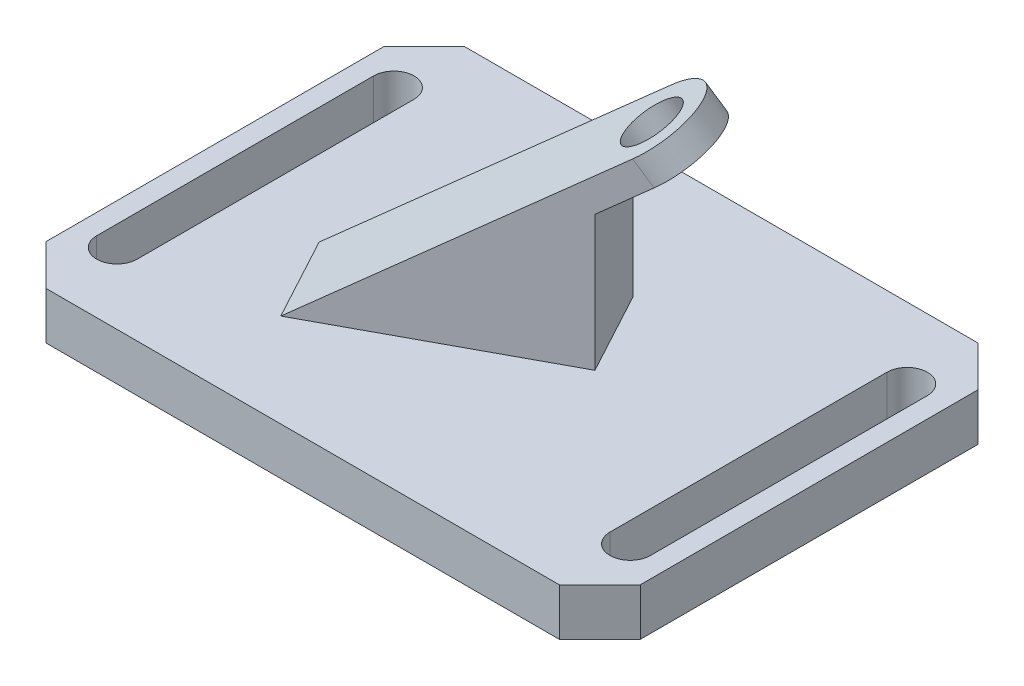
ISO-10303-21;
HEADER;
FILE_DESCRIPTION(('STEP AP214'),'2;1');
FILE_NAME('part.step','',(''),(''),'','','');
FILE_SCHEMA(('AUTOMOTIVE_DESIGN { 1 0 10303 214 1 1 1 1 }'));
ENDSEC;
DATA;
#1=APPLICATION_CONTEXT('core data for automotive mechanical design processes');
#2=APPLICATION_PROTOCOL_DEFINITION('international standard','automotive_design',2000,#1);
#3=PRODUCT_CONTEXT('',#1,'mechanical');
#4=PRODUCT('Part','Part','',(#3));
#5=PRODUCT_RELATED_PRODUCT_CATEGORY('part','',(#4));
#6=PRODUCT_DEFINITION_FORMATION('','',#4);
#7=PRODUCT_DEFINITION_CONTEXT('part definition',#1,'design');
#8=PRODUCT_DEFINITION('design','',#6,#7);
#9=PRODUCT_DEFINITION_SHAPE('','',#8);
#10=(LENGTH_UNIT() NAMED_UNIT(*) SI_UNIT(.MILLI.,.METRE.));
#11=(NAMED_UNIT(*) PLANE_ANGLE_UNIT() SI_UNIT($,.RADIAN.));
#12=(NAMED_UNIT(*) SI_UNIT($,.STERADIAN.) SOLID_ANGLE_UNIT());
#13=UNCERTAINTY_MEASURE_WITH_UNIT(LENGTH_MEASURE(1.E-05),#10,'distance_accuracy_value','');
#14=(GEOMETRIC_REPRESENTATION_CONTEXT(3) GLOBAL_UNCERTAINTY_ASSIGNED_CONTEXT((#13)) GLOBAL_UNIT_ASSIGNED_CONTEXT((#10,
#11,#12)) REPRESENTATION_CONTEXT('',''));
#15=CARTESIAN_POINT('',(0.,0.,0.));
#16=DIRECTION('',(0.,0.,1.));
#17=DIRECTION('',(1.,0.,0.));
#18=AXIS2_PLACEMENT_3D('',#15,#16,#17);
#19=CARTESIAN_POINT('',(0.,3.5,0.));
#20=DIRECTION('',(0.,-1.,0.));
#21=DIRECTION('',(0.,0.,-1.));
#22=AXIS2_PLACEMENT_3D('',#19,#20,#21);
#23=PLANE('',#22);
#24=DIRECTION('',(-0.474790242570468,0.,-0.880098986228183));
#25=VECTOR('',#24,1.);
#26=CARTESIAN_POINT('',(13.141813392465,3.5,0.863988305263869));
#27=LINE('',#26,#25);
#28=CARTESIAN_POINT('',(13.141813392465,3.5,0.863988305263869));
#29=VERTEX_POINT('',#28);
#30=CARTESIAN_POINT('',(6.49474999647841,3.5,-11.4573975019307));
#31=VERTEX_POINT('',#30);
#32=EDGE_CURVE('E59',#29,#31,#27,.T.);
#33=ORIENTED_EDGE('',*,*,#32,.F.);
#34=DIRECTION('',(0.880098986228183,0.,-0.474790242570468));
#35=VECTOR('',#34,1.);
#36=CARTESIAN_POINT('',(-17.074488577443,3.5,17.1648880521879));
#37=LINE('',#36,#35);
#38=CARTESIAN_POINT('',(-17.074488577443,3.5,17.1648880521879));
#39=VERTEX_POINT('',#38);
#40=EDGE_CURVE('E61',#39,#29,#37,.T.);
#41=ORIENTED_EDGE('',*,*,#40,.F.);
#42=DIRECTION('',(-0.474790242570468,0.,-0.880098986228183));
#43=VECTOR('',#42,1.);
#44=CARTESIAN_POINT('',(-17.074488577443,3.5,17.1648880521879));
#45=LINE('',#44,#43);
#46=CARTESIAN_POINT('',(-23.7215519734296,3.5,4.84350224499337));
#47=VERTEX_POINT('',#46);
#48=EDGE_CURVE('E228',#39,#47,#45,.T.);
#49=ORIENTED_EDGE('',*,*,#48,.T.);
#50=DIRECTION('',(0.880098986228183,0.,-0.474790242570468));
#51=VECTOR('',#50,1.);
#52=CARTESIAN_POINT('',(-23.7215519734296,3.5,4.84350224499337));
#53=LINE('',#52,#51);
#54=EDGE_CURVE('E192',#47,#31,#53,.T.);
#55=ORIENTED_EDGE('',*,*,#54,.T.);
#56=EDGE_LOOP('',(#33,#41,#49,#55));
#57=FACE_BOUND('',#56,.T.);
#58=CARTESIAN_POINT('',(-38.,3.5,20.5));
#59=DIRECTION('',(0.,1.,0.));
#60=DIRECTION('',(0.,0.,1.));
#61=AXIS2_PLACEMENT_3D('',#58,#59,#60);
#62=CIRCLE('',#61,3.);
#63=CARTESIAN_POINT('',(-41.,3.5,20.5));
#64=VERTEX_POINT('',#63);
#65=CARTESIAN_POINT('',(-35.,3.5,20.5));
#66=VERTEX_POINT('',#65);
#67=EDGE_CURVE('E268',#64,#66,#62,.T.);
#68=ORIENTED_EDGE('',*,*,#67,.F.);
#69=DIRECTION('',(0.,0.,1.));
#70=VECTOR('',#69,1.);
#71=CARTESIAN_POINT('',(-41.,3.5,20.5));
#72=LINE('',#71,#70);
#73=CARTESIAN_POINT('',(-41.,3.5,-20.5));
#74=VERTEX_POINT('',#73);
#75=EDGE_CURVE('E277',#74,#64,#72,.T.);
#76=ORIENTED_EDGE('',*,*,#75,.F.);
#77=CARTESIAN_POINT('',(-38.,3.5,-20.5));
#78=DIRECTION('',(0.,1.,0.));
#79=DIRECTION('',(0.,0.,1.));
#80=AXIS2_PLACEMENT_3D('',#77,#78,#79);
#81=CIRCLE('',#80,3.);
#82=CARTESIAN_POINT('',(-35.,3.5,-20.5));
#83=VERTEX_POINT('',#82);
#84=EDGE_CURVE('E272',#83,#74,#81,.T.);
#85=ORIENTED_EDGE('',*,*,#84,.F.);
#86=DIRECTION('',(0.,0.,-1.));
#87=VECTOR('',#86,1.);
#88=CARTESIAN_POINT('',(-35.,3.5,20.5));
#89=LINE('',#88,#87);
#90=EDGE_CURVE('E269',#66,#83,#89,.T.);
#91=ORIENTED_EDGE('',*,*,#90,.F.);
#92=EDGE_LOOP('',(#68,#76,#85,#91));
#93=FACE_BOUND('',#92,.T.);
#94=DIRECTION('',(-1.,0.,0.));
#95=VECTOR('',#94,1.);
#96=CARTESIAN_POINT('',(-38.,3.5,-31.));
#97=LINE('',#96,#95);
#98=CARTESIAN_POINT('',(38.,3.5,-31.));
#99=VERTEX_POINT('',#98);
#100=CARTESIAN_POINT('',(-38.,3.5,-31.));
#101=VERTEX_POINT('',#100);
#102=EDGE_CURVE('E299',#99,#101,#97,.T.);
#103=ORIENTED_EDGE('',*,*,#102,.T.);
#104=DIRECTION('',(-0.707106781186549,0.,0.707106781186546));
#105=VECTOR('',#104,1.);
#106=CARTESIAN_POINT('',(-44.,3.5,-25.));
#107=LINE('',#106,#105);
#108=CARTESIAN_POINT('',(-44.,3.5,-25.));
#109=VERTEX_POINT('',#108);
#110=EDGE_CURVE('E305',#101,#109,#107,.T.);
#111=ORIENTED_EDGE('',*,*,#110,.T.);
#112=DIRECTION('',(0.,0.,1.));
#113=VECTOR('',#112,1.);
#114=CARTESIAN_POINT('',(-44.,3.5,-25.));
#115=LINE('',#114,#113);
#116=CARTESIAN_POINT('',(-44.,3.5,25.));
#117=VERTEX_POINT('',#116);
#118=EDGE_CURVE('E304',#109,#117,#115,.T.);
#119=ORIENTED_EDGE('',*,*,#118,.T.);
#120=DIRECTION('',(0.707106781186547,0.,0.707106781186549));
#121=VECTOR('',#120,1.);
#122=CARTESIAN_POINT('',(-44.,3.5,25.));
#123=LINE('',#122,#121);
#124=CARTESIAN_POINT('',(-38.,3.5,31.));
#125=VERTEX_POINT('',#124);
#126=EDGE_CURVE('E307',#117,#125,#123,.T.);
#127=ORIENTED_EDGE('',*,*,#126,.T.);
#128=DIRECTION('',(1.,0.,0.));
#129=VECTOR('',#128,1.);
#130=CARTESIAN_POINT('',(-38.,3.5,31.));
#131=LINE('',#130,#129);
#132=CARTESIAN_POINT('',(38.,3.5,31.));
#133=VERTEX_POINT('',#132);
#134=EDGE_CURVE('E310',#125,#133,#131,.T.);
#135=ORIENTED_EDGE('',*,*,#134,.T.);
#136=DIRECTION('',(0.707106781186549,0.,-0.707106781186546));
#137=VECTOR('',#136,1.);
#138=CARTESIAN_POINT('',(38.,3.5,31.));
#139=LINE('',#138,#137);
#140=CARTESIAN_POINT('',(44.,3.5,25.));
#141=VERTEX_POINT('',#140);
#142=EDGE_CURVE('E313',#133,#141,#139,.T.);
#143=ORIENTED_EDGE('',*,*,#142,.T.);
#144=DIRECTION('',(0.,0.,-1.));
#145=VECTOR('',#144,1.);
#146=CARTESIAN_POINT('',(44.,3.5,-25.));
#147=LINE('',#146,#145);
#148=CARTESIAN_POINT('',(44.,3.5,-25.));
#149=VERTEX_POINT('',#148);
#150=EDGE_CURVE('E311',#141,#149,#147,.T.);
#151=ORIENTED_EDGE('',*,*,#150,.T.);
#152=DIRECTION('',(-0.707106781186549,0.,-0.707106781186547));
#153=VECTOR('',#152,1.);
#154=CARTESIAN_POINT('',(38.,3.5,-31.));
#155=LINE('',#154,#153);
#156=EDGE_CURVE('E312',#149,#99,#155,.T.);
#157=ORIENTED_EDGE('',*,*,#156,.T.);
#158=EDGE_LOOP('',(#103,#111,#119,#127,#135,#143,#151,#157));
#159=FACE_BOUND('',#158,.T.);
#160=CARTESIAN_POINT('',(38.,3.5,20.5));
#161=DIRECTION('',(0.,1.,0.));
#162=DIRECTION('',(0.,0.,-1.));
#163=AXIS2_PLACEMENT_3D('',#160,#161,#162);
#164=CIRCLE('',#163,3.);
#165=CARTESIAN_POINT('',(35.,3.5,20.5));
#166=VERTEX_POINT('',#165);
#167=CARTESIAN_POINT('',(41.,3.5,20.5));
#168=VERTEX_POINT('',#167);
#169=EDGE_CURVE('E240',#166,#168,#164,.T.);
#170=ORIENTED_EDGE('',*,*,#169,.F.);
#171=DIRECTION('',(0.,0.,1.));
#172=VECTOR('',#171,1.);
#173=CARTESIAN_POINT('',(35.,3.5,20.5));
#174=LINE('',#173,#172);
#175=CARTESIAN_POINT('',(35.,3.5,-20.5));
#176=VERTEX_POINT('',#175);
#177=EDGE_CURVE('E242',#176,#166,#174,.T.);
#178=ORIENTED_EDGE('',*,*,#177,.F.);
#179=CARTESIAN_POINT('',(38.,3.5,-20.5));
#180=DIRECTION('',(0.,1.,0.));
#181=DIRECTION('',(0.,0.,-1.));
#182=AXIS2_PLACEMENT_3D('',#179,#180,#181);
#183=CIRCLE('',#182,3.);
#184=CARTESIAN_POINT('',(41.,3.5,-20.5));
#185=VERTEX_POINT('',#184);
#186=EDGE_CURVE('E245',#185,#176,#183,.T.);
#187=ORIENTED_EDGE('',*,*,#186,.F.);
#188=DIRECTION('',(0.,0.,-1.));
#189=VECTOR('',#188,1.);
#190=CARTESIAN_POINT('',(41.,3.5,20.5));
#191=LINE('',#190,#189);
#192=EDGE_CURVE('E239',#168,#185,#191,.T.);
#193=ORIENTED_EDGE('',*,*,#192,.F.);
#194=EDGE_LOOP('',(#170,#178,#187,#193));
#195=FACE_BOUND('',#194,.T.);
#196=ADVANCED_FACE('F43',(#57,#93,#159,#195),#23,.F.);
#197=CARTESIAN_POINT('',(0.,-3.5,0.));
#198=DIRECTION('',(0.,-1.,0.));
#199=DIRECTION('',(0.,0.,-1.));
#200=AXIS2_PLACEMENT_3D('',#197,#198,#199);
#201=PLANE('',#200);
#202=DIRECTION('',(-1.,0.,0.));
#203=VECTOR('',#202,1.);
#204=CARTESIAN_POINT('',(-38.,-3.5,-31.));
#205=LINE('',#204,#203);
#206=CARTESIAN_POINT('',(38.,-3.5,-31.));
#207=VERTEX_POINT('',#206);
#208=CARTESIAN_POINT('',(-38.,-3.5,-31.));
#209=VERTEX_POINT('',#208);
#210=EDGE_CURVE('E296',#207,#209,#205,.T.);
#211=ORIENTED_EDGE('',*,*,#210,.F.);
#212=DIRECTION('',(-0.707106781186549,0.,-0.707106781186547));
#213=VECTOR('',#212,1.);
#214=CARTESIAN_POINT('',(38.,-3.5,-31.));
#215=LINE('',#214,#213);
#216=CARTESIAN_POINT('',(44.,-3.5,-25.));
#217=VERTEX_POINT('',#216);
#218=EDGE_CURVE('E302',#217,#207,#215,.T.);
#219=ORIENTED_EDGE('',*,*,#218,.F.);
#220=DIRECTION('',(0.,0.,-1.));
#221=VECTOR('',#220,1.);
#222=CARTESIAN_POINT('',(44.,-3.5,-25.));
#223=LINE('',#222,#221);
#224=CARTESIAN_POINT('',(44.,-3.5,25.));
#225=VERTEX_POINT('',#224);
#226=EDGE_CURVE('E329',#225,#217,#223,.T.);
#227=ORIENTED_EDGE('',*,*,#226,.F.);
#228=DIRECTION('',(0.707106781186549,0.,-0.707106781186546));
#229=VECTOR('',#228,1.);
#230=CARTESIAN_POINT('',(38.,-3.5,31.));
#231=LINE('',#230,#229);
#232=CARTESIAN_POINT('',(38.,-3.5,31.));
#233=VERTEX_POINT('',#232);
#234=EDGE_CURVE('E327',#233,#225,#231,.T.);
#235=ORIENTED_EDGE('',*,*,#234,.F.);
#236=DIRECTION('',(1.,0.,0.));
#237=VECTOR('',#236,1.);
#238=CARTESIAN_POINT('',(-38.,-3.5,31.));
#239=LINE('',#238,#237);
#240=CARTESIAN_POINT('',(-38.,-3.5,31.));
#241=VERTEX_POINT('',#240);
#242=EDGE_CURVE('E326',#241,#233,#239,.T.);
#243=ORIENTED_EDGE('',*,*,#242,.F.);
#244=DIRECTION('',(0.707106781186547,0.,0.707106781186549));
#245=VECTOR('',#244,1.);
#246=CARTESIAN_POINT('',(-44.,-3.5,25.));
#247=LINE('',#246,#245);
#248=CARTESIAN_POINT('',(-44.,-3.5,25.));
#249=VERTEX_POINT('',#248);
#250=EDGE_CURVE('E322',#249,#241,#247,.T.);
#251=ORIENTED_EDGE('',*,*,#250,.F.);
#252=DIRECTION('',(0.,0.,1.));
#253=VECTOR('',#252,1.);
#254=CARTESIAN_POINT('',(-44.,-3.5,-25.));
#255=LINE('',#254,#253);
#256=CARTESIAN_POINT('',(-44.,-3.5,-25.));
#257=VERTEX_POINT('',#256);
#258=EDGE_CURVE('E325',#257,#249,#255,.T.);
#259=ORIENTED_EDGE('',*,*,#258,.F.);
#260=DIRECTION('',(-0.707106781186549,0.,0.707106781186546));
#261=VECTOR('',#260,1.);
#262=CARTESIAN_POINT('',(-44.,-3.5,-25.));
#263=LINE('',#262,#261);
#264=EDGE_CURVE('E319',#209,#257,#263,.T.);
#265=ORIENTED_EDGE('',*,*,#264,.F.);
#266=EDGE_LOOP('',(#211,#219,#227,#235,#243,#251,#259,#265));
#267=FACE_BOUND('',#266,.T.);
#268=DIRECTION('',(0.,0.,1.));
#269=VECTOR('',#268,1.);
#270=CARTESIAN_POINT('',(-41.,-3.5,20.5));
#271=LINE('',#270,#269);
#272=CARTESIAN_POINT('',(-41.,-3.5,-20.5));
#273=VERTEX_POINT('',#272);
#274=CARTESIAN_POINT('',(-41.,-3.5,20.5));
#275=VERTEX_POINT('',#274);
#276=EDGE_CURVE('E271',#273,#275,#271,.T.);
#277=ORIENTED_EDGE('',*,*,#276,.T.);
#278=CARTESIAN_POINT('',(-38.,-3.5,20.5));
#279=DIRECTION('',(0.,1.,0.));
#280=DIRECTION('',(0.,0.,1.));
#281=AXIS2_PLACEMENT_3D('',#278,#279,#280);
#282=CIRCLE('',#281,3.);
#283=CARTESIAN_POINT('',(-35.,-3.5,20.5));
#284=VERTEX_POINT('',#283);
#285=EDGE_CURVE('E270',#275,#284,#282,.T.);
#286=ORIENTED_EDGE('',*,*,#285,.T.);
#287=DIRECTION('',(0.,0.,-1.));
#288=VECTOR('',#287,1.);
#289=CARTESIAN_POINT('',(-35.,-3.5,20.5));
#290=LINE('',#289,#288);
#291=CARTESIAN_POINT('',(-35.,-3.5,-20.5));
#292=VERTEX_POINT('',#291);
#293=EDGE_CURVE('E283',#284,#292,#290,.T.);
#294=ORIENTED_EDGE('',*,*,#293,.T.);
#295=CARTESIAN_POINT('',(-38.,-3.5,-20.5));
#296=DIRECTION('',(0.,1.,0.));
#297=DIRECTION('',(0.,0.,1.));
#298=AXIS2_PLACEMENT_3D('',#295,#296,#297);
#299=CIRCLE('',#298,3.);
#300=EDGE_CURVE('E284',#292,#273,#299,.T.);
#301=ORIENTED_EDGE('',*,*,#300,.T.);
#302=EDGE_LOOP('',(#277,#286,#294,#301));
#303=FACE_BOUND('',#302,.T.);
#304=DIRECTION('',(0.,0.,1.));
#305=VECTOR('',#304,1.);
#306=CARTESIAN_POINT('',(35.,-3.5,20.5));
#307=LINE('',#306,#305);
#308=CARTESIAN_POINT('',(35.,-3.5,-20.5));
#309=VERTEX_POINT('',#308);
#310=CARTESIAN_POINT('',(35.,-3.5,20.5));
#311=VERTEX_POINT('',#310);
#312=EDGE_CURVE('E238',#309,#311,#307,.T.);
#313=ORIENTED_EDGE('',*,*,#312,.T.);
#314=CARTESIAN_POINT('',(38.,-3.5,20.5));
#315=DIRECTION('',(0.,1.,0.));
#316=DIRECTION('',(0.,0.,-1.));
#317=AXIS2_PLACEMENT_3D('',#314,#315,#316);
#318=CIRCLE('',#317,3.);
#319=CARTESIAN_POINT('',(41.,-3.5,20.5));
#320=VERTEX_POINT('',#319);
#321=EDGE_CURVE('E237',#311,#320,#318,.T.);
#322=ORIENTED_EDGE('',*,*,#321,.T.);
#323=DIRECTION('',(0.,0.,-1.));
#324=VECTOR('',#323,1.);
#325=CARTESIAN_POINT('',(41.,-3.5,20.5));
#326=LINE('',#325,#324);
#327=CARTESIAN_POINT('',(41.,-3.5,-20.5));
#328=VERTEX_POINT('',#327);
#329=EDGE_CURVE('E249',#320,#328,#326,.T.);
#330=ORIENTED_EDGE('',*,*,#329,.T.);
#331=CARTESIAN_POINT('',(38.,-3.5,-20.5));
#332=DIRECTION('',(0.,1.,0.));
#333=DIRECTION('',(0.,0.,-1.));
#334=AXIS2_PLACEMENT_3D('',#331,#332,#333);
#335=CIRCLE('',#334,3.);
#336=EDGE_CURVE('E251',#328,#309,#335,.T.);
#337=ORIENTED_EDGE('',*,*,#336,.T.);
#338=EDGE_LOOP('',(#313,#322,#330,#337));
#339=FACE_BOUND('',#338,.T.);
#340=ADVANCED_FACE('F359',(#267,#303,#339),#201,.T.);
#341=CARTESIAN_POINT('',(-38.,3.5,-31.));
#342=DIRECTION('',(0.,0.,1.));
#343=DIRECTION('',(1.,0.,0.));
#344=AXIS2_PLACEMENT_3D('',#341,#342,#343);
#345=PLANE('',#344);
#346=ORIENTED_EDGE('',*,*,#210,.T.);
#347=DIRECTION('',(0.,-1.,0.));
#348=VECTOR('',#347,1.);
#349=CARTESIAN_POINT('',(-38.,3.5,-31.));
#350=LINE('',#349,#348);
#351=EDGE_CURVE('E11',#101,#209,#350,.T.);
#352=ORIENTED_EDGE('',*,*,#351,.F.);
#353=ORIENTED_EDGE('',*,*,#102,.F.);
#354=DIRECTION('',(0.,-1.,0.));
#355=VECTOR('',#354,1.);
#356=CARTESIAN_POINT('',(38.,3.5,-31.));
#357=LINE('',#356,#355);
#358=EDGE_CURVE('E320',#99,#207,#357,.T.);
#359=ORIENTED_EDGE('',*,*,#358,.T.);
#360=EDGE_LOOP('',(#346,#352,#353,#359));
#361=FACE_BOUND('',#360,.T.);
#362=ADVANCED_FACE('F44',(#361),#345,.F.);
#363=CARTESIAN_POINT('',(-44.,3.5,-25.));
#364=DIRECTION('',(0.707106781186546,0.,0.707106781186549));
#365=DIRECTION('',(0.707106781186549,0.,-0.707106781186546));
#366=AXIS2_PLACEMENT_3D('',#363,#364,#365);
#367=PLANE('',#366);
#368=ORIENTED_EDGE('',*,*,#264,.T.);
#369=DIRECTION('',(0.,-1.,0.));
#370=VECTOR('',#369,1.);
#371=CARTESIAN_POINT('',(-44.,3.5,-25.));
#372=LINE('',#371,#370);
#373=EDGE_CURVE('E51',#109,#257,#372,.T.);
#374=ORIENTED_EDGE('',*,*,#373,.F.);
#375=ORIENTED_EDGE('',*,*,#110,.F.);
#376=ORIENTED_EDGE('',*,*,#351,.T.);
#377=EDGE_LOOP('',(#368,#374,#375,#376));
#378=FACE_BOUND('',#377,.T.);
#379=ADVANCED_FACE('F378',(#378),#367,.F.);
#380=CARTESIAN_POINT('',(-44.,3.5,-25.));
#381=DIRECTION('',(1.,0.,0.));
#382=DIRECTION('',(0.,0.,-1.));
#383=AXIS2_PLACEMENT_3D('',#380,#381,#382);
#384=PLANE('',#383);
#385=ORIENTED_EDGE('',*,*,#258,.T.);
#386=DIRECTION('',(0.,-1.,0.));
#387=VECTOR('',#386,1.);
#388=CARTESIAN_POINT('',(-44.,3.5,25.));
#389=LINE('',#388,#387);
#390=EDGE_CURVE('E350',#117,#249,#389,.T.);
#391=ORIENTED_EDGE('',*,*,#390,.F.);
#392=ORIENTED_EDGE('',*,*,#118,.F.);
#393=ORIENTED_EDGE('',*,*,#373,.T.);
#394=EDGE_LOOP('',(#385,#391,#392,#393));
#395=FACE_BOUND('',#394,.T.);
#396=ADVANCED_FACE('F354',(#395),#384,.F.);
#397=CARTESIAN_POINT('',(-44.,3.5,25.));
#398=DIRECTION('',(0.707106781186548,0.,-0.707106781186546));
#399=DIRECTION('',(-0.707106781186547,0.,-0.707106781186549));
#400=AXIS2_PLACEMENT_3D('',#397,#398,#399);
#401=PLANE('',#400);
#402=ORIENTED_EDGE('',*,*,#250,.T.);
#403=DIRECTION('',(0.,-1.,0.));
#404=VECTOR('',#403,1.);
#405=CARTESIAN_POINT('',(-38.,3.5,31.));
#406=LINE('',#405,#404);
#407=EDGE_CURVE('E343',#125,#241,#406,.T.);
#408=ORIENTED_EDGE('',*,*,#407,.F.);
#409=ORIENTED_EDGE('',*,*,#126,.F.);
#410=ORIENTED_EDGE('',*,*,#390,.T.);
#411=EDGE_LOOP('',(#402,#408,#409,#410));
#412=FACE_BOUND('',#411,.T.);
#413=ADVANCED_FACE('F368',(#412),#401,.F.);
#414=CARTESIAN_POINT('',(-38.,3.5,31.));
#415=DIRECTION('',(0.,0.,-1.));
#416=DIRECTION('',(-1.,0.,0.));
#417=AXIS2_PLACEMENT_3D('',#414,#415,#416);
#418=PLANE('',#417);
#419=ORIENTED_EDGE('',*,*,#242,.T.);
#420=DIRECTION('',(0.,-1.,0.));
#421=VECTOR('',#420,1.);
#422=CARTESIAN_POINT('',(38.,3.5,31.));
#423=LINE('',#422,#421);
#424=EDGE_CURVE('E341',#133,#233,#423,.T.);
#425=ORIENTED_EDGE('',*,*,#424,.F.);
#426=ORIENTED_EDGE('',*,*,#134,.F.);
#427=ORIENTED_EDGE('',*,*,#407,.T.);
#428=EDGE_LOOP('',(#419,#425,#426,#427));
#429=FACE_BOUND('',#428,.T.);
#430=ADVANCED_FACE('F367',(#429),#418,.F.);
#431=CARTESIAN_POINT('',(38.,3.5,31.));
#432=DIRECTION('',(-0.707106781186546,0.,-0.707106781186549));
#433=DIRECTION('',(-0.707106781186549,0.,0.707106781186546));
#434=AXIS2_PLACEMENT_3D('',#431,#432,#433);
#435=PLANE('',#434);
#436=ORIENTED_EDGE('',*,*,#234,.T.);
#437=DIRECTION('',(0.,-1.,0.));
#438=VECTOR('',#437,1.);
#439=CARTESIAN_POINT('',(44.,3.5,25.));
#440=LINE('',#439,#438);
#441=EDGE_CURVE('E336',#141,#225,#440,.T.);
#442=ORIENTED_EDGE('',*,*,#441,.F.);
#443=ORIENTED_EDGE('',*,*,#142,.F.);
#444=ORIENTED_EDGE('',*,*,#424,.T.);
#445=EDGE_LOOP('',(#436,#442,#443,#444));
#446=FACE_BOUND('',#445,.T.);
#447=ADVANCED_FACE('F393',(#446),#435,.F.);
#448=CARTESIAN_POINT('',(44.,3.5,-25.));
#449=DIRECTION('',(-1.,0.,0.));
#450=DIRECTION('',(0.,0.,1.));
#451=AXIS2_PLACEMENT_3D('',#448,#449,#450);
#452=PLANE('',#451);
#453=ORIENTED_EDGE('',*,*,#226,.T.);
#454=DIRECTION('',(0.,-1.,0.));
#455=VECTOR('',#454,1.);
#456=CARTESIAN_POINT('',(44.,3.5,-25.));
#457=LINE('',#456,#455);
#458=EDGE_CURVE('E333',#149,#217,#457,.T.);
#459=ORIENTED_EDGE('',*,*,#458,.F.);
#460=ORIENTED_EDGE('',*,*,#150,.F.);
#461=ORIENTED_EDGE('',*,*,#441,.T.);
#462=EDGE_LOOP('',(#453,#459,#460,#461));
#463=FACE_BOUND('',#462,.T.);
#464=ADVANCED_FACE('F386',(#463),#452,.F.);
#465=CARTESIAN_POINT('',(38.,3.5,-31.));
#466=DIRECTION('',(-0.707106781186546,0.,0.707106781186548));
#467=DIRECTION('',(0.707106781186549,0.,0.707106781186547));
#468=AXIS2_PLACEMENT_3D('',#465,#466,#467);
#469=PLANE('',#468);
#470=ORIENTED_EDGE('',*,*,#218,.T.);
#471=ORIENTED_EDGE('',*,*,#358,.F.);
#472=ORIENTED_EDGE('',*,*,#156,.F.);
#473=ORIENTED_EDGE('',*,*,#458,.T.);
#474=EDGE_LOOP('',(#470,#471,#472,#473));
#475=FACE_BOUND('',#474,.T.);
#476=ADVANCED_FACE('F383',(#475),#469,.F.);
#477=CARTESIAN_POINT('',(-38.,3.5,20.5));
#478=DIRECTION('',(0.,-1.,0.));
#479=DIRECTION('',(0.,0.,-1.));
#480=AXIS2_PLACEMENT_3D('',#477,#478,#479);
#481=CYLINDRICAL_SURFACE('',#480,3.);
#482=ORIENTED_EDGE('',*,*,#285,.F.);
#483=DIRECTION('',(0.,-1.,0.));
#484=VECTOR('',#483,1.);
#485=CARTESIAN_POINT('',(-41.,3.5,20.5));
#486=LINE('',#485,#484);
#487=EDGE_CURVE('E279',#64,#275,#486,.T.);
#488=ORIENTED_EDGE('',*,*,#487,.F.);
#489=ORIENTED_EDGE('',*,*,#67,.T.);
#490=DIRECTION('',(0.,-1.,0.));
#491=VECTOR('',#490,1.);
#492=CARTESIAN_POINT('',(-35.,3.5,20.5));
#493=LINE('',#492,#491);
#494=EDGE_CURVE('E293',#66,#284,#493,.T.);
#495=ORIENTED_EDGE('',*,*,#494,.T.);
#496=EDGE_LOOP('',(#482,#488,#489,#495));
#497=FACE_BOUND('',#496,.T.);
#498=ADVANCED_FACE('F406',(#497),#481,.F.);
#499=CARTESIAN_POINT('',(-35.,3.5,20.5));
#500=DIRECTION('',(-1.,0.,0.));
#501=DIRECTION('',(0.,0.,1.));
#502=AXIS2_PLACEMENT_3D('',#499,#500,#501);
#503=PLANE('',#502);
#504=ORIENTED_EDGE('',*,*,#293,.F.);
#505=ORIENTED_EDGE('',*,*,#494,.F.);
#506=ORIENTED_EDGE('',*,*,#90,.T.);
#507=DIRECTION('',(0.,-1.,0.));
#508=VECTOR('',#507,1.);
#509=CARTESIAN_POINT('',(-35.,3.5,-20.5));
#510=LINE('',#509,#508);
#511=EDGE_CURVE('E291',#83,#292,#510,.T.);
#512=ORIENTED_EDGE('',*,*,#511,.T.);
#513=EDGE_LOOP('',(#504,#505,#506,#512));
#514=FACE_BOUND('',#513,.T.);
#515=ADVANCED_FACE('F414',(#514),#503,.T.);
#516=CARTESIAN_POINT('',(-38.,3.5,-20.5));
#517=DIRECTION('',(0.,-1.,0.));
#518=DIRECTION('',(0.,0.,-1.));
#519=AXIS2_PLACEMENT_3D('',#516,#517,#518);
#520=CYLINDRICAL_SURFACE('',#519,3.);
#521=ORIENTED_EDGE('',*,*,#300,.F.);
#522=ORIENTED_EDGE('',*,*,#511,.F.);
#523=ORIENTED_EDGE('',*,*,#84,.T.);
#524=DIRECTION('',(0.,-1.,0.));
#525=VECTOR('',#524,1.);
#526=CARTESIAN_POINT('',(-41.,3.5,-20.5));
#527=LINE('',#526,#525);
#528=EDGE_CURVE('E292',#74,#273,#527,.T.);
#529=ORIENTED_EDGE('',*,*,#528,.T.);
#530=EDGE_LOOP('',(#521,#522,#523,#529));
#531=FACE_BOUND('',#530,.T.);
#532=ADVANCED_FACE('F419',(#531),#520,.F.);
#533=CARTESIAN_POINT('',(-41.,3.5,20.5));
#534=DIRECTION('',(1.,0.,0.));
#535=DIRECTION('',(0.,0.,-1.));
#536=AXIS2_PLACEMENT_3D('',#533,#534,#535);
#537=PLANE('',#536);
#538=ORIENTED_EDGE('',*,*,#276,.F.);
#539=ORIENTED_EDGE('',*,*,#528,.F.);
#540=ORIENTED_EDGE('',*,*,#75,.T.);
#541=ORIENTED_EDGE('',*,*,#487,.T.);
#542=EDGE_LOOP('',(#538,#539,#540,#541));
#543=FACE_BOUND('',#542,.T.);
#544=ADVANCED_FACE('F430',(#543),#537,.T.);
#545=CARTESIAN_POINT('',(38.,3.5,20.5));
#546=DIRECTION('',(0.,-1.,0.));
#547=DIRECTION('',(0.,0.,-1.));
#548=AXIS2_PLACEMENT_3D('',#545,#546,#547);
#549=CYLINDRICAL_SURFACE('',#548,3.);
#550=ORIENTED_EDGE('',*,*,#321,.F.);
#551=DIRECTION('',(0.,-1.,0.));
#552=VECTOR('',#551,1.);
#553=CARTESIAN_POINT('',(35.,3.5,20.5));
#554=LINE('',#553,#552);
#555=EDGE_CURVE('E250',#166,#311,#554,.T.);
#556=ORIENTED_EDGE('',*,*,#555,.F.);
#557=ORIENTED_EDGE('',*,*,#169,.T.);
#558=DIRECTION('',(0.,-1.,0.));
#559=VECTOR('',#558,1.);
#560=CARTESIAN_POINT('',(41.,3.5,20.5));
#561=LINE('',#560,#559);
#562=EDGE_CURVE('E262',#168,#320,#561,.T.);
#563=ORIENTED_EDGE('',*,*,#562,.T.);
#564=EDGE_LOOP('',(#550,#556,#557,#563));
#565=FACE_BOUND('',#564,.T.);
#566=ADVANCED_FACE('F439',(#565),#549,.F.);
#567=CARTESIAN_POINT('',(41.,3.5,20.5));
#568=DIRECTION('',(-1.,0.,0.));
#569=DIRECTION('',(0.,0.,1.));
#570=AXIS2_PLACEMENT_3D('',#567,#568,#569);
#571=PLANE('',#570);
#572=ORIENTED_EDGE('',*,*,#329,.F.);
#573=ORIENTED_EDGE('',*,*,#562,.F.);
#574=ORIENTED_EDGE('',*,*,#192,.T.);
#575=DIRECTION('',(0.,-1.,0.));
#576=VECTOR('',#575,1.);
#577=CARTESIAN_POINT('',(41.,3.5,-20.5));
#578=LINE('',#577,#576);
#579=EDGE_CURVE('E265',#185,#328,#578,.T.);
#580=ORIENTED_EDGE('',*,*,#579,.T.);
#581=EDGE_LOOP('',(#572,#573,#574,#580));
#582=FACE_BOUND('',#581,.T.);
#583=ADVANCED_FACE('F443',(#582),#571,.T.);
#584=CARTESIAN_POINT('',(38.,3.5,-20.5));
#585=DIRECTION('',(0.,-1.,0.));
#586=DIRECTION('',(0.,0.,-1.));
#587=AXIS2_PLACEMENT_3D('',#584,#585,#586);
#588=CYLINDRICAL_SURFACE('',#587,3.);
#589=ORIENTED_EDGE('',*,*,#336,.F.);
#590=ORIENTED_EDGE('',*,*,#579,.F.);
#591=ORIENTED_EDGE('',*,*,#186,.T.);
#592=DIRECTION('',(0.,-1.,0.));
#593=VECTOR('',#592,1.);
#594=CARTESIAN_POINT('',(35.,3.5,-20.5));
#595=LINE('',#594,#593);
#596=EDGE_CURVE('E257',#176,#309,#595,.T.);
#597=ORIENTED_EDGE('',*,*,#596,.T.);
#598=EDGE_LOOP('',(#589,#590,#591,#597));
#599=FACE_BOUND('',#598,.T.);
#600=ADVANCED_FACE('F449',(#599),#588,.F.);
#601=CARTESIAN_POINT('',(35.,3.5,20.5));
#602=DIRECTION('',(1.,0.,0.));
#603=DIRECTION('',(0.,0.,-1.));
#604=AXIS2_PLACEMENT_3D('',#601,#602,#603);
#605=PLANE('',#604);
#606=ORIENTED_EDGE('',*,*,#312,.F.);
#607=ORIENTED_EDGE('',*,*,#596,.F.);
#608=ORIENTED_EDGE('',*,*,#177,.T.);
#609=ORIENTED_EDGE('',*,*,#555,.T.);
#610=EDGE_LOOP('',(#606,#607,#608,#609));
#611=FACE_BOUND('',#610,.T.);
#612=ADVANCED_FACE('F452',(#611),#605,.T.);
#613=CARTESIAN_POINT('',(13.141813392465,3.5,0.863988305263869));
#614=DIRECTION('',(-0.880098986228183,0.,0.474790242570468));
#615=DIRECTION('',(0.474790242570468,0.,0.880098986228183));
#616=AXIS2_PLACEMENT_3D('',#613,#614,#615);
#617=PLANE('',#616);
#618=DIRECTION('',(0.,1.,0.));
#619=VECTOR('',#618,1.);
#620=CARTESIAN_POINT('',(6.49474999647841,3.5,-11.4573975019307));
#621=LINE('',#620,#619);
#622=CARTESIAN_POINT('',(6.49474999647841,23.5,-11.4573975019307));
#623=VERTEX_POINT('',#622);
#624=EDGE_CURVE('E226',#31,#623,#621,.T.);
#625=ORIENTED_EDGE('',*,*,#624,.T.);
#626=DIRECTION('',(-0.474790242570468,0.,-0.880098986228183));
#627=VECTOR('',#626,1.);
#628=CARTESIAN_POINT('',(13.141813392465,23.5,0.863988305263869));
#629=LINE('',#628,#627);
#630=CARTESIAN_POINT('',(13.141813392465,23.5,0.863988305263869));
#631=VERTEX_POINT('',#630);
#632=EDGE_CURVE('E235',#631,#623,#629,.T.);
#633=ORIENTED_EDGE('',*,*,#632,.F.);
#634=DIRECTION('',(0.,1.,0.));
#635=VECTOR('',#634,1.);
#636=CARTESIAN_POINT('',(13.141813392465,3.5,0.863988305263869));
#637=LINE('',#636,#635);
#638=EDGE_CURVE('E218',#29,#631,#637,.T.);
#639=ORIENTED_EDGE('',*,*,#638,.F.);
#640=ORIENTED_EDGE('',*,*,#32,.T.);
#641=EDGE_LOOP('',(#625,#633,#639,#640));
#642=FACE_BOUND('',#641,.T.);
#643=ADVANCED_FACE('F460',(#642),#617,.F.);
#644=CARTESIAN_POINT('',(13.141813392465,23.5,0.863988305263869));
#645=DIRECTION('',(-0.517309204662484,0.809016994374946,0.279074702515288));
#646=DIRECTION('',(-0.842489616801312,-0.538712581607278,0.));
#647=AXIS2_PLACEMENT_3D('',#644,#645,#646);
#648=PLANE('',#647);
#649=CARTESIAN_POINT('',(15.5144019871978,28.2022820183398,-8.36961159835671));
#650=DIRECTION('',(-0.517309204662484,0.809016994374946,0.279074702515288));
#651=DIRECTION('',(-0.842489616801312,-0.538712581607278,0.));
#652=AXIS2_PLACEMENT_3D('',#649,#650,#651);
#653=CIRCLE('',#652,3.99999999999999);
#654=CARTESIAN_POINT('',(12.1444435199925,26.0474316919107,-8.36961159835671));
#655=VERTEX_POINT('',#654);
#656=EDGE_CURVE('E209',#655,#655,#653,.T.);
#657=ORIENTED_EDGE('',*,*,#656,.T.);
#658=EDGE_LOOP('',(#657));
#659=FACE_BOUND('',#658,.T.);
#660=DIRECTION('',(0.712015036590762,0.587785252292475,-0.384113375002912));
#661=VECTOR('',#660,1.);
#662=CARTESIAN_POINT('',(6.49474999647841,23.5,-11.4573975019307));
#663=LINE('',#662,#661);
#664=CARTESIAN_POINT('',(12.1908702892045,28.2022820183398,-14.530304501954));
#665=VERTEX_POINT('',#664);
#666=EDGE_CURVE('E202',#623,#665,#663,.T.);
#667=ORIENTED_EDGE('',*,*,#666,.T.);
#668=CARTESIAN_POINT('',(15.5144019871978,28.2022820183398,-8.36961159835671));
#669=DIRECTION('',(-0.517309204662484,0.809016994374946,0.279074702515288));
#670=DIRECTION('',(-0.842489616801312,-0.538712581607278,0.));
#671=AXIS2_PLACEMENT_3D('',#668,#669,#670);
#672=CIRCLE('',#671,7.);
#673=CARTESIAN_POINT('',(18.8379336851911,28.2022820183398,-2.20891869475942));
#674=VERTEX_POINT('',#673);
#675=EDGE_CURVE('E204',#674,#665,#672,.T.);
#676=ORIENTED_EDGE('',*,*,#675,.F.);
#677=DIRECTION('',(0.712015036590762,0.587785252292475,-0.384113375002912));
#678=VECTOR('',#677,1.);
#679=CARTESIAN_POINT('',(13.141813392465,23.5,0.863988305263869));
#680=LINE('',#679,#678);
#681=EDGE_CURVE('E222',#631,#674,#680,.T.);
#682=ORIENTED_EDGE('',*,*,#681,.F.);
#683=ORIENTED_EDGE('',*,*,#632,.T.);
#684=EDGE_LOOP('',(#667,#676,#682,#683));
#685=FACE_BOUND('',#684,.T.);
#686=ADVANCED_FACE('F463',(#659,#685),#648,.F.);
#687=CARTESIAN_POINT('',(-17.074488577443,3.5,17.1648880521879));
#688=DIRECTION('',(0.517309204662484,-0.809016994374946,-0.279074702515288));
#689=DIRECTION('',(0.842489616801312,0.538712581607278,0.));
#690=AXIS2_PLACEMENT_3D('',#687,#688,#689);
#691=PLANE('',#690);
#692=CARTESIAN_POINT('',(13.4451651685478,31.4383499958396,-7.25331278829556));
#693=DIRECTION('',(-0.517309204662484,0.809016994374946,0.279074702515288));
#694=DIRECTION('',(-0.842489616801312,-0.538712581607278,0.));
#695=AXIS2_PLACEMENT_3D('',#692,#693,#694);
#696=CIRCLE('',#695,3.99999999999999);
#697=CARTESIAN_POINT('',(10.0752067013426,29.2834996694105,-7.25331278829556));
#698=VERTEX_POINT('',#697);
#699=EDGE_CURVE('E212',#698,#698,#696,.T.);
#700=ORIENTED_EDGE('',*,*,#699,.F.);
#701=EDGE_LOOP('',(#700));
#702=FACE_BOUND('',#701,.T.);
#703=DIRECTION('',(-0.712015036590762,-0.587785252292475,0.384113375002912));
#704=VECTOR('',#703,1.);
#705=CARTESIAN_POINT('',(-17.074488577443,3.5,17.1648880521879));
#706=LINE('',#705,#704);
#707=CARTESIAN_POINT('',(16.7686968665411,31.4383499958396,-1.09261988469828));
#708=VERTEX_POINT('',#707);
#709=EDGE_CURVE('E207',#708,#39,#706,.T.);
#710=ORIENTED_EDGE('',*,*,#709,.F.);
#711=CARTESIAN_POINT('',(13.4451651685478,31.4383499958396,-7.25331278829556));
#712=DIRECTION('',(-0.517309204662484,0.809016994374946,0.279074702515288));
#713=DIRECTION('',(-0.842489616801312,-0.538712581607278,0.));
#714=AXIS2_PLACEMENT_3D('',#711,#712,#713);
#715=CIRCLE('',#714,7.);
#716=CARTESIAN_POINT('',(10.1216334705546,31.4383499958396,-13.4140056918928));
#717=VERTEX_POINT('',#716);
#718=EDGE_CURVE('E205',#708,#717,#715,.T.);
#719=ORIENTED_EDGE('',*,*,#718,.T.);
#720=DIRECTION('',(-0.712015036590762,-0.587785252292475,0.384113375002912));
#721=VECTOR('',#720,1.);
#722=CARTESIAN_POINT('',(-23.7215519734296,3.5,4.84350224499337));
#723=LINE('',#722,#721);
#724=EDGE_CURVE('E188',#717,#47,#723,.T.);
#725=ORIENTED_EDGE('',*,*,#724,.T.);
#726=ORIENTED_EDGE('',*,*,#48,.F.);
#727=EDGE_LOOP('',(#710,#719,#725,#726));
#728=FACE_BOUND('',#727,.T.);
#729=ADVANCED_FACE('F208',(#702,#728),#691,.F.);
#730=CARTESIAN_POINT('',(3.32353169799327,0.,6.16069290359728));
#731=DIRECTION('',(0.474790242570468,0.,0.880098986228183));
#732=DIRECTION('',(0.880098986228183,0.,-0.474790242570468));
#733=AXIS2_PLACEMENT_3D('',#730,#731,#732);
#734=PLANE('',#733);
#735=ORIENTED_EDGE('',*,*,#40,.T.);
#736=ORIENTED_EDGE('',*,*,#638,.T.);
#737=ORIENTED_EDGE('',*,*,#681,.T.);
#738=DIRECTION('',(-0.517309204662483,0.809016994374947,0.279074702515287));
#739=VECTOR('',#738,1.);
#740=CARTESIAN_POINT('',(18.8379336851911,28.2022820183398,-2.20891869475942));
#741=LINE('',#740,#739);
#742=EDGE_CURVE('E224',#674,#708,#741,.T.);
#743=ORIENTED_EDGE('',*,*,#742,.T.);
#744=ORIENTED_EDGE('',*,*,#709,.T.);
#745=EDGE_LOOP('',(#735,#736,#737,#743,#744));
#746=FACE_BOUND('',#745,.T.);
#747=ADVANCED_FACE('F467',(#746),#734,.T.);
#748=CARTESIAN_POINT('',(-3.32353169799328,0.,-6.16069290359729));
#749=DIRECTION('',(0.474790242570468,0.,0.880098986228183));
#750=DIRECTION('',(0.880098986228183,0.,-0.474790242570468));
#751=AXIS2_PLACEMENT_3D('',#748,#749,#750);
#752=PLANE('',#751);
#753=ORIENTED_EDGE('',*,*,#54,.F.);
#754=ORIENTED_EDGE('',*,*,#724,.F.);
#755=DIRECTION('',(-0.517309204662483,0.809016994374947,0.279074702515287));
#756=VECTOR('',#755,1.);
#757=CARTESIAN_POINT('',(12.1908702892045,28.2022820183398,-14.530304501954));
#758=LINE('',#757,#756);
#759=EDGE_CURVE('E187',#665,#717,#758,.T.);
#760=ORIENTED_EDGE('',*,*,#759,.F.);
#761=ORIENTED_EDGE('',*,*,#666,.F.);
#762=ORIENTED_EDGE('',*,*,#624,.F.);
#763=EDGE_LOOP('',(#753,#754,#760,#761,#762));
#764=FACE_BOUND('',#763,.T.);
#765=ADVANCED_FACE('F186',(#764),#752,.F.);
#766=CARTESIAN_POINT('',(15.5144019871978,28.2022820183398,-8.36961159835671));
#767=DIRECTION('',(-0.517309204662484,0.809016994374946,0.279074702515288));
#768=DIRECTION('',(-0.842489616801312,-0.538712581607278,0.));
#769=AXIS2_PLACEMENT_3D('',#766,#767,#768);
#770=CYLINDRICAL_SURFACE('',#769,7.);
#771=ORIENTED_EDGE('',*,*,#742,.F.);
#772=ORIENTED_EDGE('',*,*,#675,.T.);
#773=ORIENTED_EDGE('',*,*,#759,.T.);
#774=ORIENTED_EDGE('',*,*,#718,.F.);
#775=EDGE_LOOP('',(#771,#772,#773,#774));
#776=FACE_BOUND('',#775,.T.);
#777=ADVANCED_FACE('F203',(#776),#770,.T.);
#778=CARTESIAN_POINT('',(15.5144019871978,28.2022820183398,-8.36961159835671));
#779=DIRECTION('',(-0.517309204662484,0.809016994374946,0.279074702515288));
#780=DIRECTION('',(-0.842489616801312,-0.538712581607278,0.));
#781=AXIS2_PLACEMENT_3D('',#778,#779,#780);
#782=CYLINDRICAL_SURFACE('',#781,3.99999999999999);
#783=ORIENTED_EDGE('',*,*,#656,.F.);
#784=EDGE_LOOP('',(#783));
#785=FACE_BOUND('',#784,.T.);
#786=ORIENTED_EDGE('',*,*,#699,.T.);
#787=EDGE_LOOP('',(#786));
#788=FACE_BOUND('',#787,.T.);
#789=ADVANCED_FACE('F480',(#785,#788),#782,.F.);
#790=CLOSED_SHELL('',(#196,#340,#362,#379,#396,#413,#430,#447,#464,#476,#498,#515,#532,#544,
#566,#583,#600,#612,#643,#686,#729,#747,#765,#777,#789));
#791=MANIFOLD_SOLID_BREP('B2',#790);
#792=ADVANCED_BREP_SHAPE_REPRESENTATION('',(#18,#791),#14);
#793=SHAPE_DEFINITION_REPRESENTATION(#9,#792);
ENDSEC;
END-ISO-10303-21;
